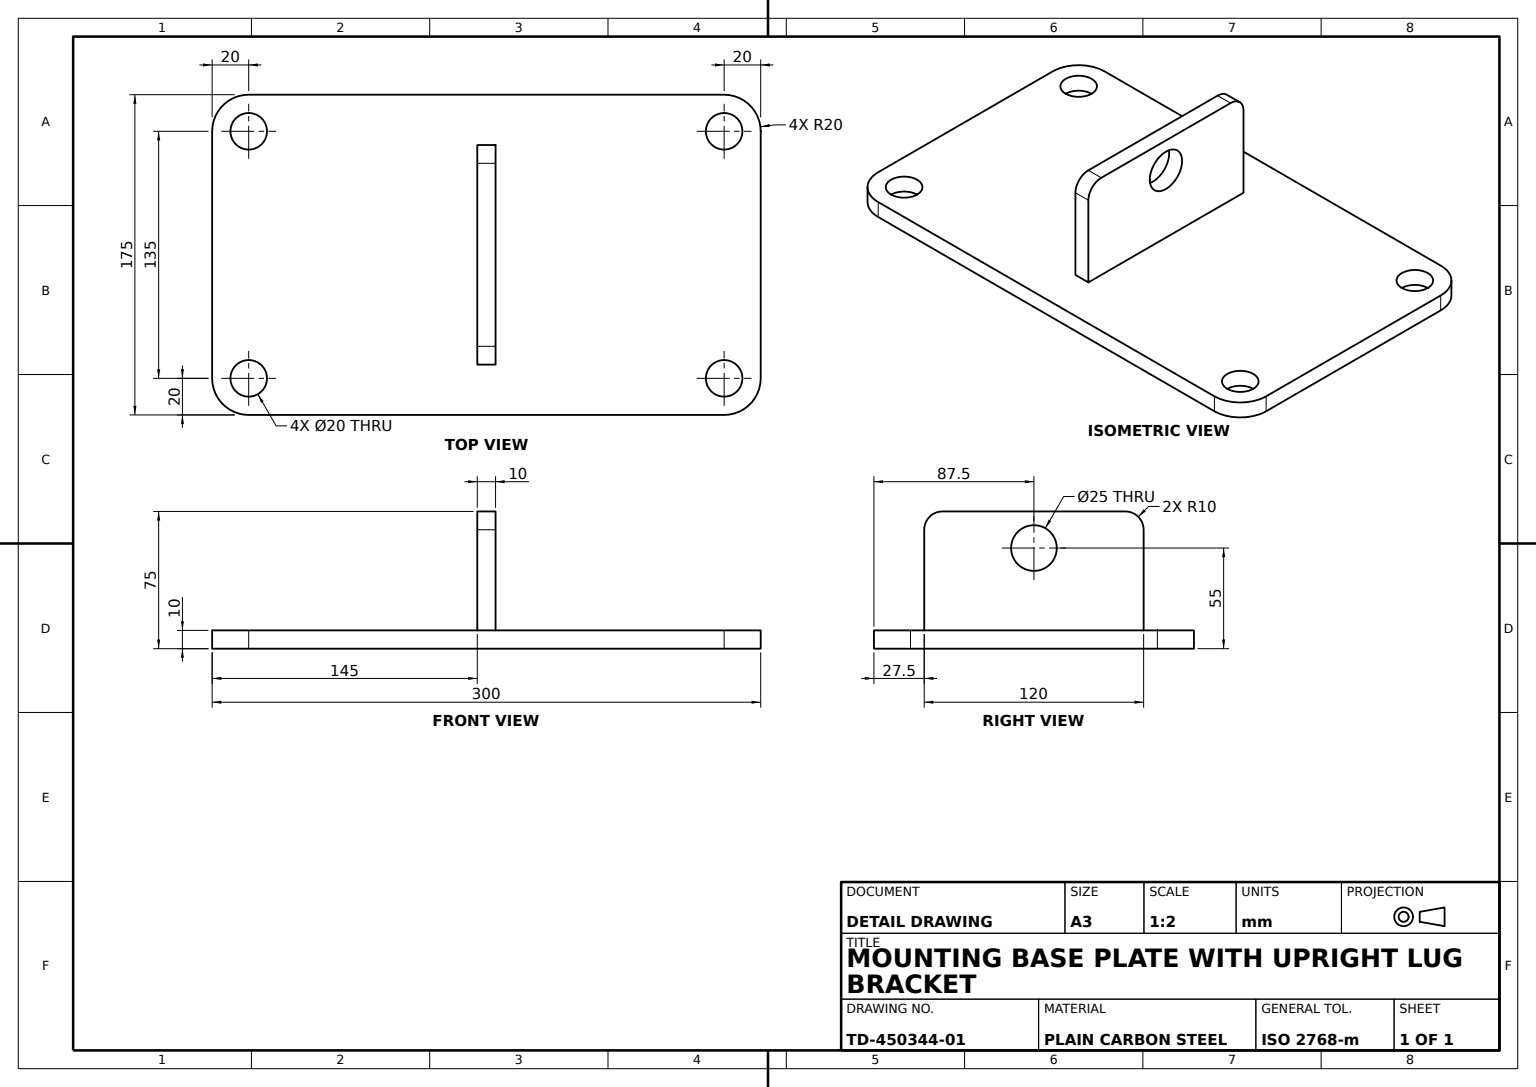
SolidWorks part; units mm, degrees
material "Plain Carbon Steel"
ref_plane "Front Plane" through (0, 0, 0) normal (0, 0, 1) x (1, 0, 0)
ref_plane "Top Plane" through (0, 0, 0) normal (0, 1, 0) x (1, 0, 0)
ref_plane "Right Plane" through (0, 0, 0) normal (1, 0, 0) x (0, 0, -1)
sketch "Base Plate Sketch" plane through (0, 0, 0) normal (0, 1, 0) x (1, 0, 0)
  line L1 (-130, -87.5) -> (130, -87.5)
  line L2 (-150, -67.5) -> (-150, 67.5)
  line L3 (-130, 87.5) -> (130, 87.5)
  line L4 (150, -67.5) -> (150, 67.5)
  arc A0 (150, 67.5) -> (130, 87.5) centre (130, 67.5) ccw
  arc A1 (130, -87.5) -> (150, -67.5) centre (130, -67.5) ccw
  arc A2 (-130, -87.5) -> (-150, -67.5) centre (-130, -67.5) cw
  arc A3 (-150, 67.5) -> (-130, 87.5) centre (-130, 67.5) cw
  point P0 (0, 0)
  dimension "D3" = 20
  dimension "D1" = 150
  dimension "D2" = 300
  dimension "D4" = 87.5
  dimension "D5" = 175
extrude "Base Plate" add sketch "Base Plate Sketch" along normal blind 10
sketch "Mounting Holes Sketch" plane through (0, 10, 0) normal (0, 1, 0) x (1, 0, 0)
  circle A1 centre (130, 67.5) radius 10
  circle A2 centre (130, -67.5) radius 10
  circle A4 centre (-130, 67.5) radius 10
  circle A5 centre (-130, -67.5) radius 10
  dimension "D1" = 20
  dimension "D2" = 20
  dimension "D3" = 20
  dimension "D4" = 20
extrude "Mounting Holes 4x" cut sketch "Mounting Holes Sketch" against normal blind 10
sketch "Upright Tab Sketch" plane through (0, 10, 0) normal (0, 1, 0) x (1, 0, 0)
  line L1 (-5, -60) -> (5, -60)
  line L2 (-5, -60) -> (-5, 60)
  line L3 (-5, 60) -> (5, 60)
  line L4 (5, -60) -> (5, 60)
  line L5 (-5, -60) -> (5, 60) construction
  line L6 (-5, 60) -> (5, -60) construction
  point P0 (0, 0)
  point P10 (0, -60)
  dimension "D1" = 10
  dimension "D2" = 120
extrude "Upright Tab" add sketch "Upright Tab Sketch" along normal blind 65
fillet "Tab Corner Fillet 1 R10" radius 10 1 edges at (0, 75, 60)
fillet "Tab Corner Fillet 2 R10" radius 10 1 edges at (0, 75, -60)
sketch "Tab Hole Sketch" plane through (5, 0, 0) normal (1, 0, 0) x (0, 0, -1)
  line L0 (-67.5, 0) -> (67.5, 0) construction
  circle A0 centre (0, 55) radius 12.5
  dimension "D1" = 25
  dimension "D2" = 55
  dimension "D3" = 60
extrude "Tab Hole" cut sketch "Tab Hole Sketch" against normal blind 65
